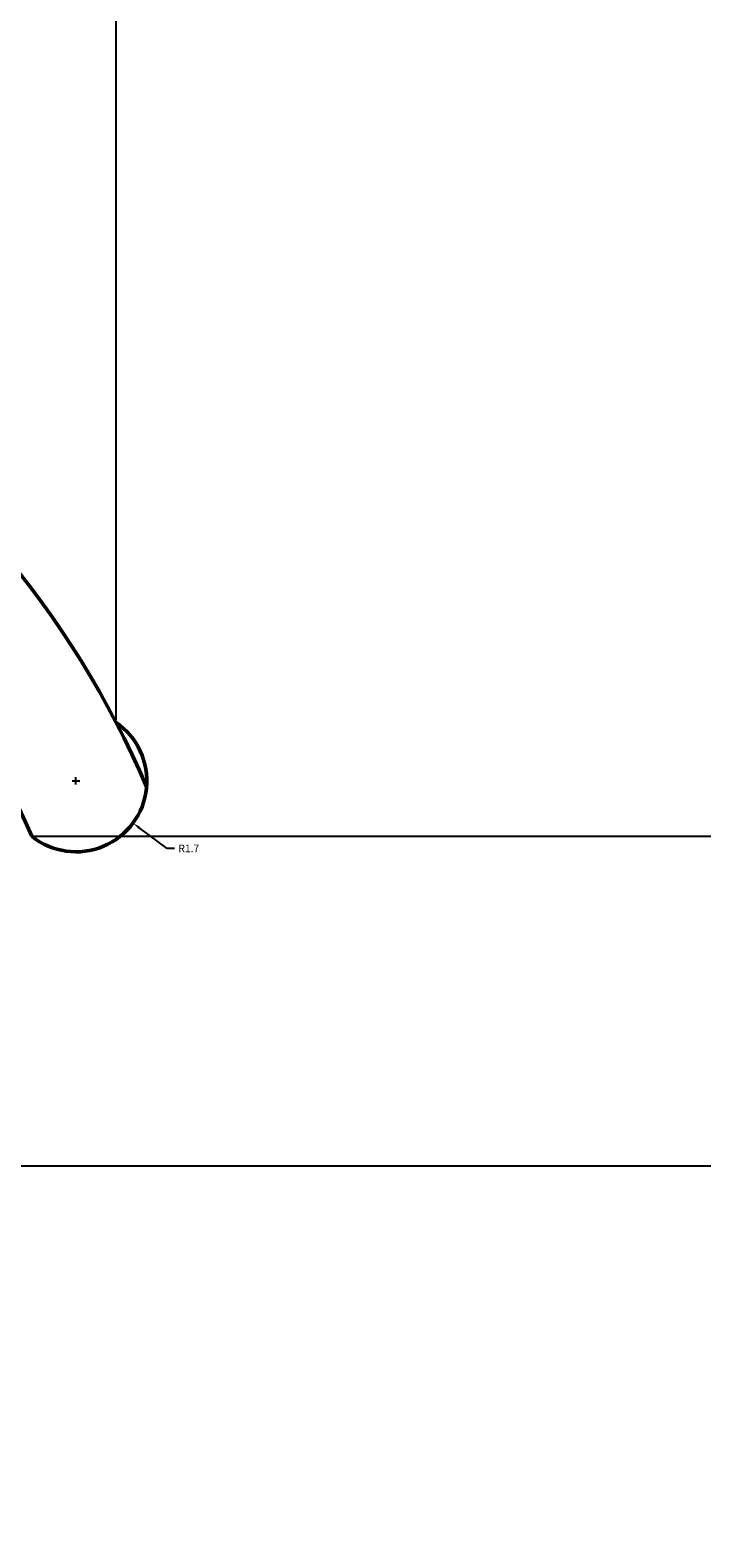
# Model space of a CAD drawing. Units: inches. Extents: x -14 to 108, y -9 to 83.
# Tile 11 of 13: x 65 to 82, y 28 to 64. Entities that reach past the tile are written whole.
import ezdxf

# ---------------------------------------------------------------- set-up
doc = ezdxf.new("R2010")
doc.units = ezdxf.units.IN
doc.header["$MEASUREMENT"] = 0
doc.layers.add('M-DIMS', color=2, linetype='Continuous', lineweight=18)
doc.layers.add('M-OUTL', color=7, linetype='Continuous', lineweight=50)
doc.styles.get("Standard").update_dxf_attribs({"font": 'arial.ttf'})
doc.dimstyles.get("Standard").update_dxf_attribs({"dimtxt": 0.18, "dimasz": 0.18, "dimexe": 0.18, "dimexo": 0.0625, "dimgap": 0.09, "dimtad": 0, "dimtih": 1, "dimtoh": 1, "dimzin": 0, "dimdsep": 46, "dimtxsty": 'Standard', "dimcen": 0.09, "dimadec": 0, "dimazin": 0, "dimtfac": 1, "dimtofl": 0, "dimtmove": 0, "dimatfit": 3, "dimfxl": 1, "dimtolj": 1, "dimtzin": 0, "dimarcsym": 0})

# ---------------------------------------------------------------- blocks, each defined once
blk = doc.blocks.new('*D8')
at = {"layer": 'Defpoints', "color": 0, "transparency": 16777216}
for p in [(47.098, 37.119), (81.545, 18.227), (81.545, -8.596)]:
    blk.add_point(p, dxfattribs=at)
at = {"layer": 'M-DIMS', "color": 0, "lineweight": -2, "transparency": 16777216}
for p, q in [((47.098, 37.057), (47.098, -8.776)), ((81.545, 18.165), (81.545, -8.776)), ((47.278, -8.596), (63.927, -8.596)), ((81.365, -8.596), (64.716, -8.596))]:
    blk.add_line(p, q, dxfattribs=at)
at = {"layer": 'M-DIMS', "color": 0, "transparency": 16777216}
for points in [[(47.278, -8.566), (47.278, -8.626), (47.098, -8.596)], [(81.365, -8.566), (81.365, -8.626), (81.545, -8.596)]]:
    blk.add_solid(points, dxfattribs=at)
at = {"layer": 'M-DIMS', "color": 0, "transparency": 16777216, "insert": (64.321, -8.596), "char_height": 0.18, "attachment_point": 5}
blk.add_mtext('\\A1;34.45', dxfattribs=at)
blk = doc.blocks.new('*D11')
at = {"layer": 'Defpoints', "color": 0, "transparency": 16777216}
for p in [(47.098, 37.119), (107.813, 37.119), (86.478, 18.227)]:
    blk.add_point(p, dxfattribs=at)
at = {"layer": 'M-DIMS', "color": 0, "lineweight": -2, "transparency": 16777216}
for p, q in [((47.16, 37.119), (107.993, 37.119)), ((107.813, 36.939), (107.813, 27.855)), ((107.813, 18.407), (107.813, 27.491)), ((86.541, 18.227), (107.993, 18.227))]:
    blk.add_line(p, q, dxfattribs=at)
at = {"layer": 'M-DIMS', "color": 0, "transparency": 16777216}
for points in [[(107.783, 36.939), (107.843, 36.939), (107.813, 37.119)], [(107.783, 18.407), (107.843, 18.407), (107.813, 18.227)]]:
    blk.add_solid(points, dxfattribs=at)
at = {"layer": 'M-DIMS', "color": 0, "transparency": 16777216, "insert": (107.813, 27.673), "char_height": 0.18, "attachment_point": 5}
blk.add_mtext('\\A1;18.892', dxfattribs=at)
blk = doc.blocks.new('*D12')
at = {"layer": 'Defpoints', "color": 0, "transparency": 16777216}
for p in [(86.478, 57.664), (107.813, 57.664), (47.098, 37.119)]:
    blk.add_point(p, dxfattribs=at)
at = {"layer": 'M-DIMS', "color": 0, "lineweight": -2, "transparency": 16777216}
for p, q in [((86.541, 57.664), (107.993, 57.664)), ((107.813, 57.484), (107.813, 47.573)), ((107.813, 37.299), (107.813, 47.21)), ((47.16, 37.119), (107.993, 37.119))]:
    blk.add_line(p, q, dxfattribs=at)
at = {"layer": 'M-DIMS', "color": 0, "transparency": 16777216}
for points in [[(107.783, 57.484), (107.843, 57.484), (107.813, 57.664)], [(107.783, 37.299), (107.843, 37.299), (107.813, 37.119)]]:
    blk.add_solid(points, dxfattribs=at)
at = {"layer": 'M-DIMS', "color": 0, "transparency": 16777216, "insert": (107.813, 47.392), "char_height": 0.18, "attachment_point": 5}
blk.add_mtext('\\A1;20.544', dxfattribs=at)
blk = doc.blocks.new('*D21')
at = {"layer": 'Defpoints', "color": 0, "transparency": 16777216}
for p in [(65.47, 45.024), (107.813, 45.024), (47.098, 37.119)]:
    blk.add_point(p, dxfattribs=at)
at = {"layer": 'M-DIMS', "color": 0, "lineweight": -2, "transparency": 16777216}
for p, q in [((65.532, 45.024), (107.993, 45.024)), ((107.813, 44.844), (107.813, 41.254)), ((107.813, 37.299), (107.813, 40.89)), ((47.16, 37.119), (107.993, 37.119))]:
    blk.add_line(p, q, dxfattribs=at)
at = {"layer": 'M-DIMS', "color": 0, "transparency": 16777216}
for points in [[(107.783, 44.844), (107.843, 44.844), (107.813, 45.024)], [(107.783, 37.299), (107.843, 37.299), (107.813, 37.119)]]:
    blk.add_solid(points, dxfattribs=at)
at = {"layer": 'M-DIMS', "color": 0, "transparency": 16777216, "insert": (107.813, 41.072), "char_height": 0.18, "attachment_point": 5}
blk.add_mtext('\\A1;7.905', dxfattribs=at)
blk = doc.blocks.new('*D22')
at = {"layer": 'Defpoints', "color": 0, "transparency": 16777216}
for p in [(67.492, 82.834), (47.098, 60.119), (67.492, 47.754)]:
    blk.add_point(p, dxfattribs=at)
at = {"layer": 'M-DIMS', "color": 0, "lineweight": -2, "transparency": 16777216}
for p, q in [((47.098, 60.182), (47.098, 83.014)), ((47.278, 82.834), (56.83, 82.834)), ((67.312, 82.834), (57.76, 82.834)), ((67.492, 47.817), (67.492, 83.014))]:
    blk.add_line(p, q, dxfattribs=at)
at = {"layer": 'M-DIMS', "color": 0, "transparency": 16777216}
for points in [[(47.278, 82.864), (47.278, 82.804), (47.098, 82.834)], [(67.312, 82.864), (67.312, 82.804), (67.492, 82.834)]]:
    blk.add_solid(points, dxfattribs=at)
at = {"layer": 'M-DIMS', "color": 0, "transparency": 16777216, "insert": (57.295, 82.834), "char_height": 0.18, "attachment_point": 5}
blk.add_mtext('\\A1;20.394', dxfattribs=at)
blk = doc.blocks.new('*D30')
at = {"layer": 'Defpoints', "color": 0, "transparency": 16777216}
for p in [(59.745, 56.33), (47.098, 37.119)]:
    blk.add_point(p, dxfattribs=at)
at = {"layer": 'M-DIMS', "color": 0, "lineweight": -2, "transparency": 16777216}
for p, q in [((67.333, 67.856), (59.844, 56.48)), ((67.513, 67.856), (67.333, 67.856)), ((47.008, 37.119), (47.188, 37.119)), ((47.098, 37.029), (47.098, 37.209))]:
    blk.add_line(p, q, dxfattribs=at)
at = {"layer": 'M-DIMS', "color": 0, "transparency": 16777216}
blk.add_solid([(59.819, 56.497), (59.869, 56.464), (59.745, 56.33)], dxfattribs=at)
at = {"layer": 'M-DIMS', "color": 0, "transparency": 16777216, "insert": (67.818, 67.856), "char_height": 0.18, "attachment_point": 5}
blk.add_mtext('\\A1;R23', dxfattribs=at)
blk = doc.blocks.new('*D33')
at = {"layer": 'Defpoints', "color": 0, "transparency": 16777216}
for p in [(66.531, 46.352), (67.897, 45.34)]:
    blk.add_point(p, dxfattribs=at)
at = {"layer": 'M-DIMS', "color": 0, "lineweight": -2, "transparency": 16777216}
for p, q in [((66.441, 46.352), (66.621, 46.352)), ((66.531, 46.262), (66.531, 46.442)), ((68.717, 44.733), (68.042, 45.233)), ((68.897, 44.733), (68.717, 44.733))]:
    blk.add_line(p, q, dxfattribs=at)
at = {"layer": 'M-DIMS', "color": 0, "transparency": 16777216}
blk.add_solid([(68.06, 45.257), (68.024, 45.209), (67.897, 45.34)], dxfattribs=at)
at = {"layer": 'M-DIMS', "color": 0, "transparency": 16777216, "insert": (69.237, 44.733), "char_height": 0.18, "attachment_point": 5}
blk.add_mtext('\\A1;R1.7', dxfattribs=at)

msp = doc.modelspace()

# ---------------------------------------------------------------- linework, layer by layer
at = {"layer": 'M-OUTL'}
for centre, radius, start, end in [((47.0979, 37.1193), 23, 23.2807, 90), ((47.0979, 37.1193), 20, 23.2807, 90), ((66.5313, 46.3515), 1.6999, 231.34463, 55.605)]:
    msp.add_arc(centre, radius, start, end, dxfattribs=at)

# ---------------------------------------------------------------- dimensions: what is measured, and where the dimension line sits
at = {"layer": 'M-DIMS'}
for base, p1, p2, override, picture, middle in [((67.4915, 82.8343), (47.0979, 60.1193), (67.4915, 47.7542), {"dimdec": 3, "dimlfac": 1, "dimrnd": 0, "dimzin": 0, "dimdsep": 46, "dimlunit": 2}, '*D22', (57.2947, 82.8343)), ((81.5446, -8.5957), (47.0979, 37.1193), (81.5446, 18.2274), {"dimdec": 2, "dimlfac": 1, "dimrnd": 0, "dimzin": 0, "dimdsep": 46, "dimlunit": 2}, '*D8', (64.3213, -8.5957))]:
    dim = msp.add_linear_dim(base=base, p1=p1, p2=p2, dimstyle='Standard', override=override, dxfattribs=at)
    dim.commit()
    dim.dimension.update_dxf_attribs({"geometry": picture, "text_midpoint": middle})
for center, mpoint, override, picture, middle in [((47.0979, 37.1193), (59.745, 56.33), {"dimdec": 0, "dimlfac": 1, "dimrnd": 0, "dimzin": 0, "dimdsep": 46, "dimlunit": 2}, '*D30', (67.8183, 67.8564)), ((66.5313, 46.3515), (67.8973, 45.3398), {"dimdec": 1, "dimlfac": 1, "dimrnd": 0, "dimzin": 0, "dimdsep": 46, "dimlunit": 2}, '*D33', (69.2369, 44.7327))]:
    dim = msp.add_radius_dim(center=center, mpoint=mpoint, dimstyle='Standard', override=override, dxfattribs=at)
    dim.commit()
    dim.dimension.update_dxf_attribs({"geometry": picture, "text_midpoint": middle, "dimtype": 164})
for base, p1, p2, picture, middle in [((107.8129, 57.6637), (47.0979, 37.1193), (86.4784, 57.6637), '*D12', (107.8129, 47.3915)), ((107.8129, 45.0241), (47.0979, 37.1193), (65.4695, 45.0241), '*D21', (107.8129, 41.0717)), ((107.8129, 37.1193), (86.4784, 18.2274), (47.0979, 37.1193), '*D11', (107.8129, 27.6733))]:
    dim = msp.add_linear_dim(base=base, p1=p1, p2=p2, angle=90, dimstyle='Standard', override={"dimdec": 3, "dimlfac": 1, "dimrnd": 0, "dimzin": 0, "dimdsep": 46, "dimlunit": 2}, dxfattribs=at)
    dim.commit()
    dim.dimension.update_dxf_attribs({"geometry": picture, "text_midpoint": middle})

doc.saveas('drawing.dxf')
